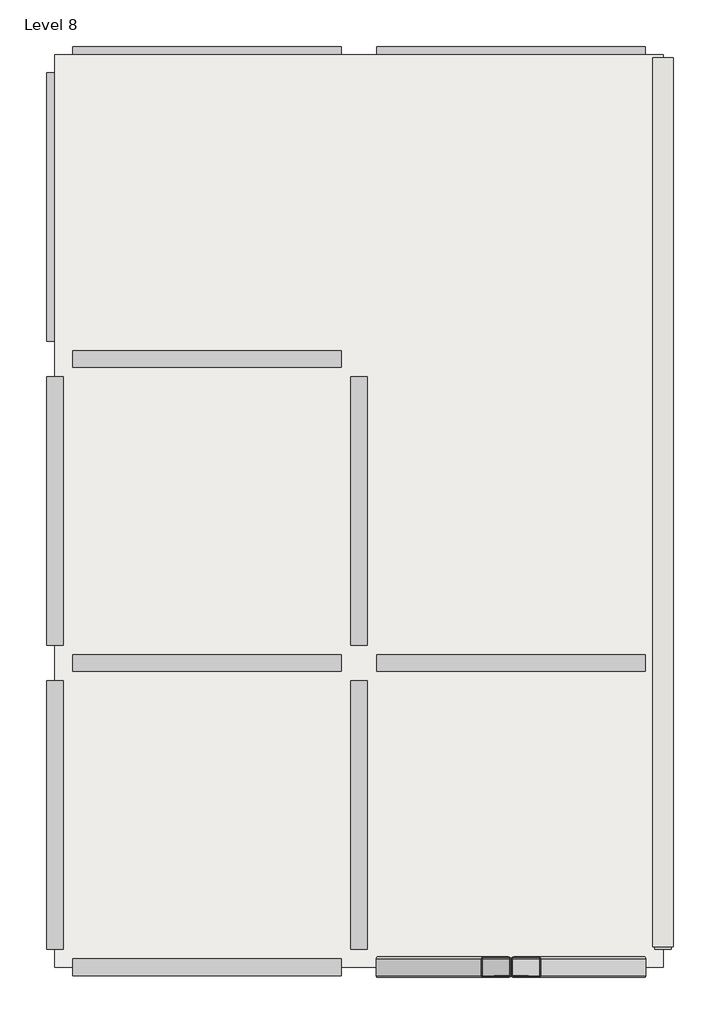
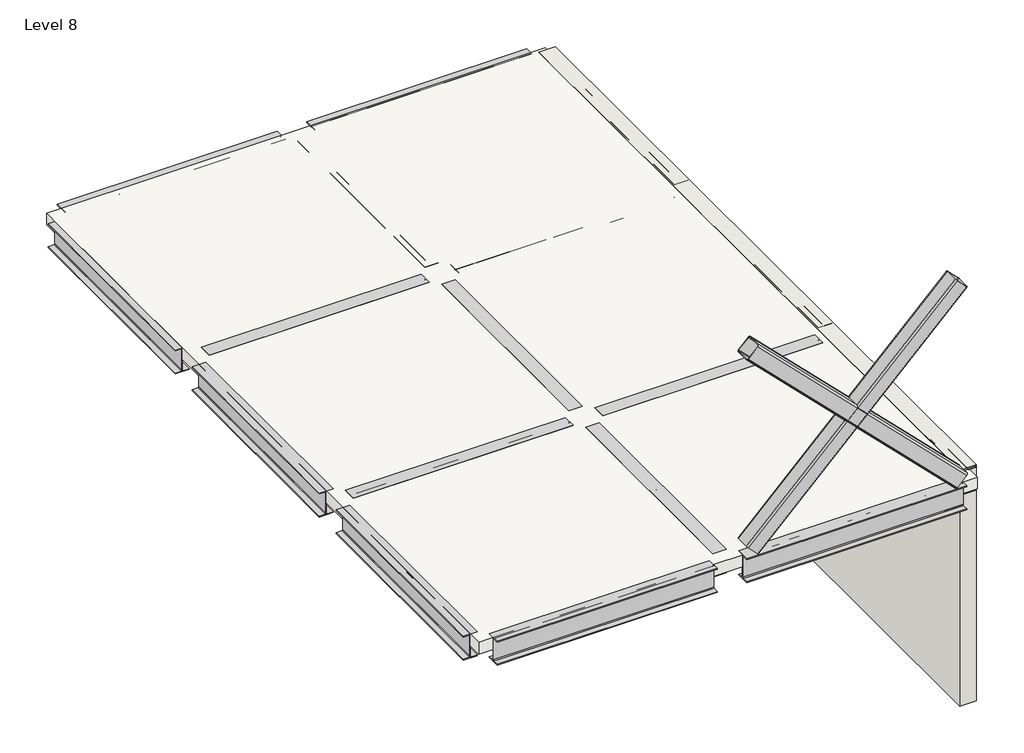
# One storey: 17 beams, 2 members, 1 slab, 1 wall.
"""IFC4 building model written with IfcOpenShell, lengths in millimetres."""

from ifc_helpers import new_model, si_unit, frame, origin, place, context, project, spatial, polyline, outline, extrude, transform, mapped, element, save
from components import ub_universal_beams_ub305x165x40_60ab2ee1, m_hss_square_hss203_2x203_2x9_5_07d005dd

model = new_model("IFC4")

# Units and contexts
model_context = context("Model", 3, world=origin())
ifc_project = project(units=[si_unit("LENGTHUNIT", "METRE", prefix="MILLI")], contexts=[model_context])

# Site, building, storey
site = spatial("IfcSite", under=ifc_project)
building = spatial("IfcBuilding", under=site)
storey = spatial("IfcBuildingStorey", under=building, Name="Level 8", Elevation=21000.0)

# Beams
placement = place(None, origin())
ub_universal_beams_ub305x165x40_shape = ub_universal_beams_ub305x165x40_60ab2ee1(model_context)
element("IfcBeam", 1, ObjectType="UB-Universal Beams : UB305x165x40", at=placement, inside=storey, context=model_context, shape_type="MappedRepresentation", body=[
    mapped(ub_universal_beams_ub305x165x40_shape, transform((18435.1404262, -6314.7314166, 20848.3), x_axis=(-1.0, 0.0, 0.0), y_axis=(0.0, -1.0, 0.0), z_axis=(0.0, 0.0, 1.0))),
])
element("IfcBeam", 2, ObjectType="UB-Universal Beams : UB305x165x40", at=placement, inside=storey, context=model_context, shape_type="MappedRepresentation", body=[
    mapped(ub_universal_beams_ub305x165x40_shape, transform((15435.1404262, -6314.7314166, 20848.3), x_axis=(-1.0, 0.0, 0.0), y_axis=(0.0, -1.0, 0.0), z_axis=(0.0, 0.0, 1.0))),
])
element("IfcBeam", 3, ObjectType="UB-Universal Beams : UB305x165x40", at=placement, inside=storey, context=model_context, shape_type="MappedRepresentation", body=[
    mapped(ub_universal_beams_ub305x165x40_shape, transform((13935.1404262, -4814.7314166, 20848.3), x_axis=(0.0, 1.0, 0.0), y_axis=(-1.0, 0.0, 0.0), z_axis=(0.0, 0.0, 1.0))),
])
element("IfcBeam", 4, ObjectType="UB-Universal Beams : UB305x165x40", at=placement, inside=storey, context=model_context, shape_type="MappedRepresentation", body=[
    mapped(ub_universal_beams_ub305x165x40_shape, transform((13935.1404262, -1814.7314166, 20848.3), x_axis=(0.0, 1.0, 0.0), y_axis=(-1.0, 0.0, 0.0), z_axis=(0.0, 0.0, 1.0))),
])
element("IfcBeam", 5, ObjectType="UB-Universal Beams : UB305x165x40", at=placement, inside=storey, context=model_context, shape_type="MappedRepresentation", body=[
    mapped(ub_universal_beams_ub305x165x40_shape, transform((13935.1404262, 1185.2685834, 20848.3), x_axis=(0.0, 1.0, 0.0), y_axis=(-1.0, 0.0, 0.0), z_axis=(0.0, 0.0, 1.0))),
])
element("IfcBeam", 6, ObjectType="UB-Universal Beams : UB305x165x40", at=placement, inside=storey, context=model_context, shape_type="MappedRepresentation", body=[
    mapped(ub_universal_beams_ub305x165x40_shape, transform((18435.1404262, -3314.7314166, 20848.3), x_axis=(-1.0, 0.0, 0.0), y_axis=(0.0, -1.0, 0.0), z_axis=(0.0, 0.0, 1.0))),
])
element("IfcBeam", 7, ObjectType="UB-Universal Beams : UB305x165x40", at=placement, inside=storey, context=model_context, shape_type="MappedRepresentation", body=[
    mapped(ub_universal_beams_ub305x165x40_shape, transform((15435.1404262, -3314.7314166, 20848.3), x_axis=(-1.0, 0.0, 0.0), y_axis=(0.0, -1.0, 0.0), z_axis=(0.0, 0.0, 1.0))),
])
element("IfcBeam", 8, ObjectType="UB-Universal Beams : UB305x165x40", at=placement, inside=storey, context=model_context, shape_type="MappedRepresentation", body=[
    mapped(ub_universal_beams_ub305x165x40_shape, transform((18435.1404262, -314.7314166, 20848.3), x_axis=(-1.0, 0.0, 0.0), y_axis=(0.0, -1.0, 0.0), z_axis=(0.0, 0.0, 1.0))),
])
element("IfcBeam", 9, ObjectType="UB-Universal Beams : UB305x165x40", at=placement, inside=storey, context=model_context, shape_type="MappedRepresentation", body=[
    mapped(ub_universal_beams_ub305x165x40_shape, transform((15435.1404262, -314.7314166, 20848.3), x_axis=(-1.0, 0.0, 0.0), y_axis=(0.0, -1.0, 0.0), z_axis=(0.0, 0.0, 1.0))),
])
element("IfcBeam", 10, ObjectType="UB-Universal Beams : UB305x165x40", at=placement, inside=storey, context=model_context, shape_type="MappedRepresentation", body=[
    mapped(ub_universal_beams_ub305x165x40_shape, transform((18435.1404262, 2685.2685834, 20848.3), x_axis=(-1.0, 0.0, 0.0), y_axis=(0.0, -1.0, 0.0), z_axis=(0.0, 0.0, 1.0))),
])
element("IfcBeam", 11, ObjectType="UB-Universal Beams : UB305x165x40", at=placement, inside=storey, context=model_context, shape_type="MappedRepresentation", body=[
    mapped(ub_universal_beams_ub305x165x40_shape, transform((15435.1404262, 2685.2685834, 20848.3), x_axis=(-1.0, 0.0, 0.0), y_axis=(0.0, -1.0, 0.0), z_axis=(0.0, 0.0, 1.0))),
])
element("IfcBeam", 12, ObjectType="UB-Universal Beams : UB305x165x40", at=placement, inside=storey, context=model_context, shape_type="MappedRepresentation", body=[
    mapped(ub_universal_beams_ub305x165x40_shape, transform((16935.1404262, -4814.7314166, 20848.3), x_axis=(0.0, 1.0, 0.0), y_axis=(-1.0, 0.0, 0.0), z_axis=(0.0, 0.0, 1.0))),
])
element("IfcBeam", 13, ObjectType="UB-Universal Beams : UB305x165x40", at=placement, inside=storey, context=model_context, shape_type="MappedRepresentation", body=[
    mapped(ub_universal_beams_ub305x165x40_shape, transform((16935.1404262, -1814.7314166, 20848.3), x_axis=(0.0, 1.0, 0.0), y_axis=(-1.0, 0.0, 0.0), z_axis=(0.0, 0.0, 1.0))),
])
element("IfcBeam", 14, ObjectType="UB-Universal Beams : UB305x165x40", at=placement, inside=storey, context=model_context, shape_type="MappedRepresentation", body=[
    mapped(ub_universal_beams_ub305x165x40_shape, transform((16935.1404262, 1185.2685834, 20848.3), x_axis=(0.0, 1.0, 0.0), y_axis=(-1.0, 0.0, 0.0), z_axis=(0.0, 0.0, 1.0))),
])
element("IfcBeam", 15, ObjectType="UB-Universal Beams : UB305x165x40", at=placement, inside=storey, context=model_context, shape_type="MappedRepresentation", body=[
    mapped(ub_universal_beams_ub305x165x40_shape, transform((19935.1404262, -1814.7314166, 20848.3), x_axis=(0.0, 1.0, 0.0), y_axis=(-1.0, 0.0, 0.0), z_axis=(0.0, 0.0, 1.0))),
])
element("IfcBeam", 16, ObjectType="UB-Universal Beams : UB305x165x40", at=placement, inside=storey, context=model_context, shape_type="MappedRepresentation", body=[
    mapped(ub_universal_beams_ub305x165x40_shape, transform((19935.1404262, 1185.2685834, 20848.3), x_axis=(0.0, 1.0, 0.0), y_axis=(-1.0, 0.0, 0.0), z_axis=(0.0, 0.0, 1.0))),
])
element("IfcBeam", 17, ObjectType="UB-Universal Beams : beam", at=placement, inside=storey, context=model_context, shape_type="MappedRepresentation", body=[
    mapped(ub_universal_beams_ub305x165x40_shape, transform((19935.1404262, -4814.7314166, 20848.3), x_axis=(0.0, 1.0, 0.0), y_axis=(-1.0, 0.0, 0.0), z_axis=(0.0, 0.0, 1.0))),
])

# Members
m_hss_square_hss203_2x203_2x9_5_shape = m_hss_square_hss203_2x203_2x9_5_07d005dd(model_context)
element("IfcMember", 18, ObjectType="M_HSS Square : HSS203.2X203.2X9.5", at=placement, inside=storey, context=model_context, shape_type="MappedRepresentation", body=[
    mapped(m_hss_square_hss203_2x203_2x9_5_shape, transform((18435.1404262, -6314.7314166, 22348.3), x_axis=(-0.7071067811865478, 0.0, 0.7071067811865476), y_axis=(0.0, -1.0000000000000002, 0.0), z_axis=(0.7071067811865476, 0.0, 0.7071067811865478))),
])
element("IfcMember", 19, ObjectType="M_HSS Square : HSS203.2X203.2X9.5", at=placement, inside=storey, context=model_context, shape_type="MappedRepresentation", body=[
    mapped(m_hss_square_hss203_2x203_2x9_5_shape, transform((18435.1404262, -6314.7314166, 22348.3), x_axis=(-0.7071067811865478, 0.0, -0.7071067811865475), y_axis=(0.0, -1.0000000000000002, 0.0), z_axis=(-0.7071067811865475, 0.0, 0.7071067811865478))),
])

# Slab
element("IfcSlab", 20, ObjectType="150mm Foundation Slab", at=placement, inside=storey, context=model_context, shape_type="SweptSolid", body=[
    extrude(outline(polyline([(13935.1404262, -6314.7314166), (13935.1404262, 2685.2685834), (19935.1404262, 2685.2685834), (19935.1404262, -6314.7314166), (13935.1404262, -6314.7314166)])), frame((0.0, 0.0, 20850.0), z_axis=(0.0, 0.0, 1.0), x_axis=(1.0, 0.0, 0.0)), (0.0, 0.0, 1.0), 150.0),
])

# Wall
element("IfcWall", 21, ObjectType="Generic - 200mm", at=placement, inside=storey, context=model_context, shape_type="SweptSolid", body=[
    extrude(outline(polyline([(19835.1404262, -6114.7314166), (19835.1404262, 2655.9792615), (20035.1404262, 2655.9792615), (20035.1404262, -6114.7314166), (19835.1404262, -6114.7314166)])), frame((0.0, 0.0, 18000.0), z_axis=(0.0, 0.0, 1.0), x_axis=(1.0, 0.0, 0.0)), (0.0, 0.0, 1.0), 3000.0),
])

save(model, "model.ifc")

# Revit data of these elements
# Type "UB-Universal Beams : UB305x165x40"
#   Section Name Key = "UB305X165X40"
#   Width = 16.5 cm
#   Web Thickness = 0.6 cm
#   Web Fillet = 0.89 cm
#   Warping Constant = 164000.0 cm⁶
#   Torsional Moment of Inertia = 14.70 cm⁴
#   Section Area = 51.3 cm²
#   Plastic Modulus weak axis = 142.0 cm³
#   Plastic Modulus strong axis = 623.0 cm³
#   Nominal Weight = 40.2999 kgf/m
#   Moment of Inertia weak axis = 764.00 cm⁴
#   Moment of Inertia strong axis = 8503.00 cm⁴
#   Height = 30.34 cm
#   Flange Thickness = 1.02 cm
#   Elastic Modulus weak axis = 92.6 cm³
#   Elastic Modulus strong axis = 560.0 cm³
#   Centroid Vertical = 15.17 cm
#   Centroid Horizontal = 8.25 cm
#   Bolt Spacing = 9.0 cm
#   Length [instance default] = 1.5 m
#   Structural Material [instance default] = Metal - Steel 43-275
#   Type Comments = ""
#   Assembly Code = ""
# Type "UB-Universal Beams : beam"
#   Section Name Key = "UB305X165X40"
#   Width = 16.5 cm
#   Web Thickness = 0.6 cm
#   Web Fillet = 0.89 cm
#   Warping Constant = 164000.0 cm⁶
#   Torsional Moment of Inertia = 14.70 cm⁴
#   Section Area = 51.3 cm²
#   Plastic Modulus weak axis = 142.0 cm³
#   Plastic Modulus strong axis = 623.0 cm³
#   Nominal Weight = 40.2999 kgf/m
#   Moment of Inertia weak axis = 764.00 cm⁴
#   Moment of Inertia strong axis = 8503.00 cm⁴
#   Height = 30.34 cm
#   Flange Thickness = 1.02 cm
#   Elastic Modulus weak axis = 92.6 cm³
#   Elastic Modulus strong axis = 560.0 cm³
#   Centroid Vertical = 15.17 cm
#   Centroid Horizontal = 8.25 cm
#   Bolt Spacing = 9.0 cm
#   Length [instance default] = 1.5 m
#   Structural Material [instance default] = Metal - Steel 43-275
#   Type Comments = ""
#   Assembly Code = ""
# Type "M_HSS Square : HSS203.2X203.2X9.5"
#   Section Name Key = "HSS 8X8X3/8"
#   Width = 20.3 cm
#   Wall Nominal Thickness = 0.953 cm
#   Wall Design Thickness = 0.886 cm
#   Torsional Moment of Inertia = 6660.00 cm⁴
#   Torsional Modulus = 10930171.7 cm³
#   Section Area = 67.1 cm²
#   Plastic Modulus weak axis = 482.0 cm³
#   Plastic Modulus strong axis = 482.0 cm³
#   Outer Fillet = 1.906 cm
#   Nominal Weight = 55.9998 kgf/m
#   Moment of Inertia weak axis = 4160.00 cm⁴
#   Moment of Inertia strong axis = 4160.00 cm⁴
#   Length [instance default] = 1.524 m
#   Inner Fillet = 0.953 cm
#   Height = 20.3 cm
#   Elastic Modulus weak axis = 408.0 cm³
#   Elastic Modulus strong axis = 408.0 cm³
#   Centroid Vertical = 10.15 cm
#   Centroid Horizontal = 10.15 cm
#   Structural Material [instance default] = Steel, 45-345
# Type "150mm Foundation Slab"
#   Layers, outside or top first: 0.15 m "Concrete, Cast-in-Place gray" (function 1)
# Type "Generic - 200mm"
#   Layers, outside or top first: 0.2 m no material (function 1)
# Elements 1, 2, 3, 4, 5, 6, 7, 8, 9, 10, 11, 12, 13, 14, 15, 16 (IfcBeam, "UB-Universal Beams : UB305x165x40")
#   Structural Material = Metal - Steel 43-275
#   Phase Created = New Construction
#   Materials on its faces: "Metal - Steel 43-275"
# Element 17 (IfcBeam, "UB-Universal Beams : beam")
#   Structural Material = Metal - Steel 43-275
#   Phase Created = New Construction
#   Materials on its faces: "Metal - Steel 43-275"
# Elements 18, 19 (IfcMember, "M_HSS Square : HSS203.2X203.2X9.5")
#   Comments = ""
#   Structural Material = Metal - Steel 43-275
#   Phase Created = New Construction
#   Materials on its faces: "Metal - Steel 43-275"
# Element 20 (IfcSlab, "150mm Foundation Slab")
#   built-in parameter 1001955 = 3.14159 (stored number, unit not read)
#   Height Offset From Level = 0 m
#   built-in parameter 1001954 = 1
#   Phase Created = New Construction
#   Materials on its faces: "Concrete, Cast-in-Place gray"
# Element 21 (IfcWall, "Generic - 200mm")
#   Comments = ""
#   built-in parameter 1001111 = -3 m
#   Top Offset = 0 m
#   Base Offset = -3 m
#   wall height = 3 m
#   Phase Created = New Construction
#   Base Constraint = Level 8
#   Top Constraint = Level 8
#   Materials on its faces: "Default Wall"
# Materials
#   "Metal - Steel 43-275": class "Metal", colour RGB 247 247 247, transparency 0, Cost = 0
#   "Steel, 45-345": class "Metal", colour RGB 247 247 247, transparency 0, Description = "Steel 345 MPa", Cost = 0
#   "Concrete, Cast-in-Place gray": class "Concrete", colour RGB 192 192 192, transparency 0, Description = "Cast-in-place concrete", Cost = 0
#   "Default Wall": colour RGB 128 128 128, transparency 0, Cost = 0
